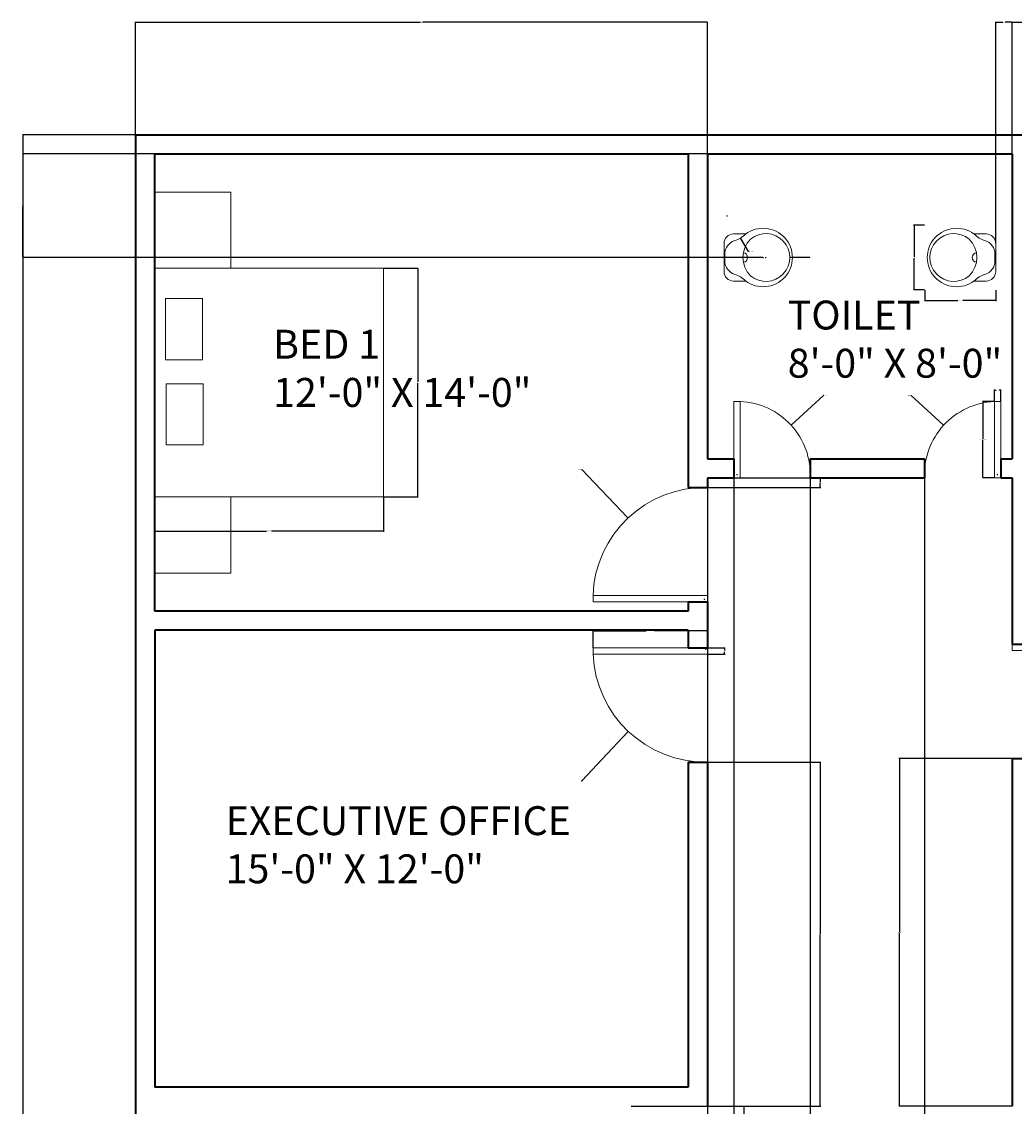
# Model space of a CAD drawing. Units: inches. Extents: x 4468 to 4972, y 2758 to 3538.
# Tile 3 of 4: x 4468 to 4781, y 3196 to 3538. Entities that reach past the tile are written whole.
import ezdxf

# ---------------------------------------------------------------- set-up
doc = ezdxf.new("R2010")
doc.units = ezdxf.units.IN
for name, color, linetype, lineweight in [('A-ANNO-DIMS', 2, 'Continuous', 18), ('A-AREA-IDEN', 7, 'Continuous', 18), ('A-DOOR', 4, 'Continuous', 18), ('A-FLOR-FIXT', 9, 'Continuous', 18), ('A-FURN', 8, 'Continuous', 15), ('A-WALL', 7, 'Continuous', 35)]:
    doc.layers.add(name, color=color, linetype=linetype, lineweight=lineweight)
doc.styles.get("Standard").update_dxf_attribs({"font": 'arial.ttf'})
doc.dimstyles.get("Standard").update_dxf_attribs({"dimtxt": 0.18, "dimasz": 0.18, "dimexe": 0.18, "dimexo": 0.0625, "dimgap": 0.09, "dimtad": 0, "dimtih": 1, "dimtoh": 1, "dimdec": 4, "dimzin": 0, "dimdsep": 46, "dimtxsty": 'Standard', "dimcen": 0.09, "dimadec": 0, "dimazin": 0, "dimtfac": 1, "dimtdec": 4, "dimtofl": 0, "dimtmove": 0, "dimatfit": 3, "dimfxl": 1, "dimtolj": 1, "dimtzin": 0, "dimarcsym": 0})

# ---------------------------------------------------------------- blocks, each defined once
blk = doc.blocks.new('A$C6EF51710')
at = {"linetype": 'ByBlock'}
for p, q in [((0.0508, 0.2843), (0.1169, 0.2843)), ((0, 0.0811), (0, 0.2335)), ((0.0041, 0.1392), (0.0041, 0.1755)), ((0.1169, 0.0303), (0.0508, 0.0303))]:
    blk.add_line(p, q, dxfattribs=at)
for centre, radius, start, end in [((0.2107, 0.1573), 0.1576, 232.89836, 127.10164), ((0.0508, 0.2335), 0.0508, 90, 180), ((0.0803, 0.1755), 0.0762, 107.10464, 180), ((0.0168, 0.3818), 0.1397, 287.10464, 315), ((0.2413, 0.1573), 0.1397, 135, 225), ((0.2254, 0.1573), 0.1289, 230.00836, 129.99164), ((0.1016, 0.1573), 0.0254, 275.21591, 84.78409), ((0.0803, 0.1392), 0.0762, 180, 252.89536), ((0.0508, 0.0811), 0.0508, 180, 270), ((0.0168, -0.0672), 0.1397, 45, 72.89536)]:
    blk.add_arc(centre, radius, start, end, dxfattribs=at)
blk = doc.blocks.new('DOOR-LEAF-36IN')
for p, q in [((0, 0), (0, 36)), ((0, 36), (2, 36)), ((2, 36), (2, 0)), ((2, 0), (0, 0))]:
    blk.add_line(p, q)
blk = doc.blocks.new('DOOR-LEAF-24IN')
for p, q in [((2, 24), (0, 24)), ((0, 24), (0, 0)), ((2, 0), (2, 24)), ((0, 0), (2, 0))]:
    blk.add_line(p, q)
blk = doc.blocks.new('BED-FRAME-72X72')
for p, q in [((0, 72), (0, 0)), ((0, 72), (72, 72)), ((0, 0), (72, 0))]:
    blk.add_line(p, q)
blk = doc.blocks.new('BED-PILLOW-PAIR')
for points in [[(0, 46.15), (11.65, 46.15), (11.65, 26.85), (0, 26.85)], [(0.18, 19.3), (11.83, 19.3), (11.83, 0), (0.18, 0)]]:
    blk.add_lwpolyline(points, close=True)
blk = doc.blocks.new('NIGHTSTAND-24X24')
blk.add_lwpolyline([(24, 24), (24, 0), (0, 0), (0, 24)], close=True)
blk = doc.blocks.new('*D17')
at = {"layer": 'A-ANNO-DIMS', "color": 0, "lineweight": -2, "transparency": 16777216}
for p, q in [((4648.18, 3340.62), (4648.18, 3346.13)), ((4648.36, 3345.95), (4664.89, 3345.95)), ((4684, 3345.95), (4667.46, 3345.95)), ((4684.18, 3340.62), (4684.18, 3346.13))]:
    blk.add_line(p, q, dxfattribs=at)
at = {"layer": 'A-ANNO-DIMS', "color": 0, "transparency": 16777216}
for points in [[(4648.36, 3345.98), (4648.36, 3345.92), (4648.18, 3345.95)], [(4684, 3345.98), (4684, 3345.92), (4684.18, 3345.95)]]:
    blk.add_solid(points, dxfattribs=at)
at = {"layer": 'Defpoints', "color": 0, "transparency": 16777216}
for p in [(4684.18, 3345.95), (4648.18, 3340.55), (4684.18, 3340.55)]:
    blk.add_point(p, dxfattribs=at)
at = {"layer": 'A-ANNO-DIMS', "color": 0, "transparency": 16777216, "insert": (4666.18, 3345.95), "char_height": 0.18, "attachment_point": 5}
blk.add_mtext('\\A1;DOOR LEAF 36 TYP.', dxfattribs=at)
blk = doc.blocks.new('*D18')
at = {"layer": 'A-ANNO-DIMS', "color": 0, "lineweight": -2, "transparency": 16777216}
for p, q in [((4684.24, 3340.55), (4689.76, 3340.55)), ((4684.24, 3338.55), (4689.76, 3338.55)), ((4689.58, 3340.37), (4689.58, 3339.73)), ((4689.58, 3338.73), (4689.58, 3339.37))]:
    blk.add_line(p, q, dxfattribs=at)
at = {"layer": 'A-ANNO-DIMS', "color": 0, "transparency": 16777216}
for points in [[(4689.55, 3340.37), (4689.61, 3340.37), (4689.58, 3340.55)], [(4689.55, 3338.73), (4689.61, 3338.73), (4689.58, 3338.55)]]:
    blk.add_solid(points, dxfattribs=at)
at = {"layer": 'Defpoints', "color": 0, "transparency": 16777216}
for p in [(4684.18, 3340.55), (4684.18, 3338.55), (4689.58, 3338.55)]:
    blk.add_point(p, dxfattribs=at)
at = {"layer": 'A-ANNO-DIMS', "color": 0, "transparency": 16777216, "insert": (4689.58, 3339.55), "char_height": 0.18, "attachment_point": 5}
blk.add_mtext('\\A1;2 TYP.', dxfattribs=at)
blk = doc.blocks.new('*D25')
at = {"layer": 'A-ANNO-DIMS', "color": 0, "lineweight": -2, "transparency": 16777216}
for p, q in [((4752.63, 3453.27), (4752.63, 3449.8)), ((4774.97, 3453.27), (4774.97, 3449.8)), ((4752.81, 3449.98), (4763.03, 3449.98)), ((4774.79, 3449.98), (4764.58, 3449.98))]:
    blk.add_line(p, q, dxfattribs=at)
at = {"layer": 'A-ANNO-DIMS', "color": 0, "transparency": 16777216}
for points in [[(4752.81, 3450.01), (4752.81, 3449.95), (4752.63, 3449.98)], [(4774.79, 3450.01), (4774.79, 3449.95), (4774.97, 3449.98)]]:
    blk.add_solid(points, dxfattribs=at)
at = {"layer": 'Defpoints', "color": 0, "transparency": 16777216}
for p in [(4752.63, 3453.33), (4774.97, 3453.33), (4752.63, 3449.98)]:
    blk.add_point(p, dxfattribs=at)
at = {"layer": 'A-ANNO-DIMS', "color": 0, "transparency": 16777216, "insert": (4763.8, 3449.98), "char_height": 0.18, "attachment_point": 5}
blk.add_mtext('\\A1;WC 22 TYP.', dxfattribs=at)
blk = doc.blocks.new('*D26')
at = {"layer": 'A-ANNO-DIMS', "color": 0, "lineweight": -2, "transparency": 16777216}
for p, q in [((4752.57, 3473.78), (4749.1, 3473.78)), ((4749.28, 3473.6), (4749.28, 3463.74)), ((4749.28, 3453.51), (4749.28, 3463.37)), ((4752.57, 3453.33), (4749.1, 3453.33))]:
    blk.add_line(p, q, dxfattribs=at)
at = {"layer": 'A-ANNO-DIMS', "color": 0, "transparency": 16777216}
for points in [[(4749.25, 3473.6), (4749.31, 3473.6), (4749.28, 3473.78)], [(4749.25, 3453.51), (4749.31, 3453.51), (4749.28, 3453.33)]]:
    blk.add_solid(points, dxfattribs=at)
at = {"layer": 'Defpoints', "color": 0, "transparency": 16777216}
for p in [(4749.28, 3473.78), (4752.63, 3473.78), (4752.63, 3453.33)]:
    blk.add_point(p, dxfattribs=at)
at = {"layer": 'A-ANNO-DIMS', "color": 0, "transparency": 16777216, "insert": (4749.28, 3463.55), "char_height": 0.18, "attachment_point": 5}
blk.add_mtext('\\A1;20 TYP.', dxfattribs=at)
blk = doc.blocks.new('*D29')
at = {"layer": 'A-ANNO-DIMS', "color": 0, "lineweight": -2, "transparency": 16777216}
for p, q in [((4774.49, 3418.16), (4770.77, 3418.16)), ((4770.95, 3417.98), (4770.95, 3406.34)), ((4770.95, 3394.34), (4770.95, 3405.98)), ((4774.49, 3394.16), (4770.77, 3394.16))]:
    blk.add_line(p, q, dxfattribs=at)
at = {"layer": 'A-ANNO-DIMS', "color": 0, "transparency": 16777216}
for points in [[(4770.92, 3417.98), (4770.98, 3417.98), (4770.95, 3418.16)], [(4770.92, 3394.34), (4770.98, 3394.34), (4770.95, 3394.16)]]:
    blk.add_solid(points, dxfattribs=at)
at = {"layer": 'Defpoints', "color": 0, "transparency": 16777216}
for p in [(4770.95, 3418.16), (4774.55, 3418.16), (4774.55, 3394.16)]:
    blk.add_point(p, dxfattribs=at)
at = {"layer": 'A-ANNO-DIMS', "color": 0, "transparency": 16777216, "insert": (4770.95, 3406.16), "char_height": 0.18, "attachment_point": 5}
blk.add_mtext('\\A1;DOOR LEAF 24 TYP.', dxfattribs=at)
blk = doc.blocks.new('*D30')
at = {"layer": 'A-ANNO-DIMS', "color": 0, "lineweight": -2, "transparency": 16777216}
for p, q in [((4774.55, 3418.22), (4774.55, 3421.94)), ((4774.73, 3421.76), (4775.09, 3421.76)), ((4776.37, 3421.76), (4776.01, 3421.76)), ((4776.55, 3418.22), (4776.55, 3421.94))]:
    blk.add_line(p, q, dxfattribs=at)
at = {"layer": 'A-ANNO-DIMS', "color": 0, "transparency": 16777216}
for points in [[(4774.73, 3421.79), (4774.73, 3421.73), (4774.55, 3421.76)], [(4776.37, 3421.79), (4776.37, 3421.73), (4776.55, 3421.76)]]:
    blk.add_solid(points, dxfattribs=at)
at = {"layer": 'Defpoints', "color": 0, "transparency": 16777216}
for p in [(4776.55, 3421.76), (4774.55, 3418.16), (4776.55, 3418.16)]:
    blk.add_point(p, dxfattribs=at)
at = {"layer": 'A-ANNO-DIMS', "color": 0, "transparency": 16777216, "insert": (4775.55, 3421.76), "char_height": 0.18, "attachment_point": 5}
blk.add_mtext('\\A1;2 TYP.', dxfattribs=at)
blk = doc.blocks.new('*D31')
at = {"layer": 'A-ANNO-DIMS', "color": 0, "lineweight": -2, "transparency": 16777216}
for p, q in [((4510.18, 3388.1), (4510.18, 3377.18)), ((4582.18, 3388.1), (4582.18, 3377.18)), ((4510.36, 3377.36), (4545.36, 3377.36)), ((4582, 3377.36), (4546.99, 3377.36))]:
    blk.add_line(p, q, dxfattribs=at)
at = {"layer": 'A-ANNO-DIMS', "color": 0, "transparency": 16777216}
for points in [[(4510.36, 3377.39), (4510.36, 3377.33), (4510.18, 3377.36)], [(4582, 3377.39), (4582, 3377.33), (4582.18, 3377.36)]]:
    blk.add_solid(points, dxfattribs=at)
at = {"layer": 'Defpoints', "color": 0, "transparency": 16777216}
for p in [(4510.18, 3388.16), (4582.18, 3388.16), (4510.18, 3377.36)]:
    blk.add_point(p, dxfattribs=at)
at = {"layer": 'A-ANNO-DIMS', "color": 0, "transparency": 16777216, "insert": (4546.18, 3377.36), "char_height": 0.18, "attachment_point": 5}
blk.add_mtext('\\A1;BED 72 TYP.', dxfattribs=at)
blk = doc.blocks.new('*D32')
at = {"layer": 'A-ANNO-DIMS', "color": 0, "lineweight": -2, "transparency": 16777216}
for p, q in [((4582.24, 3460.16), (4593.16, 3460.16)), ((4592.98, 3459.98), (4592.98, 3424.34)), ((4592.98, 3388.34), (4592.98, 3423.98)), ((4582.24, 3388.16), (4593.16, 3388.16))]:
    blk.add_line(p, q, dxfattribs=at)
at = {"layer": 'A-ANNO-DIMS', "color": 0, "transparency": 16777216}
for points in [[(4592.95, 3459.98), (4593.01, 3459.98), (4592.98, 3460.16)], [(4592.95, 3388.34), (4593.01, 3388.34), (4592.98, 3388.16)]]:
    blk.add_solid(points, dxfattribs=at)
at = {"layer": 'Defpoints', "color": 0, "transparency": 16777216}
for p in [(4582.18, 3460.16), (4582.18, 3388.16), (4592.98, 3388.16)]:
    blk.add_point(p, dxfattribs=at)
at = {"layer": 'A-ANNO-DIMS', "color": 0, "transparency": 16777216, "insert": (4592.98, 3424.16), "char_height": 0.18, "attachment_point": 5}
blk.add_mtext('\\A1;72 TYP.', dxfattribs=at)
blk = doc.blocks.new('*D38')
at = {"layer": 'A-ANNO-DIMS', "color": 0, "lineweight": -2, "transparency": 16777216}
for p, q in [((4504.11, 3502.16), (4468.5, 3502.16)), ((4468.68, 3501.98), (4468.68, 3148.34)), ((4468.68, 2794.34), (4468.68, 3147.98)), ((4780.11, 2794.16), (4468.5, 2794.16))]:
    blk.add_line(p, q, dxfattribs=at)
at = {"layer": 'A-ANNO-DIMS', "color": 0, "transparency": 16777216}
for points in [[(4468.65, 3501.98), (4468.71, 3501.98), (4468.68, 3502.16)], [(4468.65, 2794.34), (4468.71, 2794.34), (4468.68, 2794.16)]]:
    blk.add_solid(points, dxfattribs=at)
at = {"layer": 'Defpoints', "color": 0, "transparency": 16777216}
for p in [(4468.68, 3502.16), (4504.18, 3502.16), (4780.18, 2794.16)]:
    blk.add_point(p, dxfattribs=at)
at = {"layer": 'A-ANNO-DIMS', "color": 0, "transparency": 16777216, "insert": (4468.68, 3148.16), "char_height": 0.18, "attachment_point": 5}
blk.add_mtext('\\A1;708', dxfattribs=at)
blk = doc.blocks.new('*D39')
at = {"layer": 'A-ANNO-DIMS', "color": 0, "lineweight": -2, "transparency": 16777216}
for p, q in [((4504.18, 3502.22), (4504.18, 3537.84)), ((4504.36, 3537.66), (4593.9, 3537.66)), ((4684, 3537.66), (4594.46, 3537.66)), ((4684.18, 3496.22), (4684.18, 3537.84))]:
    blk.add_line(p, q, dxfattribs=at)
at = {"layer": 'A-ANNO-DIMS', "color": 0, "transparency": 16777216}
for points in [[(4504.36, 3537.69), (4504.36, 3537.63), (4504.18, 3537.66)], [(4684, 3537.69), (4684, 3537.63), (4684.18, 3537.66)]]:
    blk.add_solid(points, dxfattribs=at)
at = {"layer": 'Defpoints', "color": 0, "transparency": 16777216}
for p in [(4684.18, 3537.66), (4504.18, 3502.16), (4684.18, 3496.16)]:
    blk.add_point(p, dxfattribs=at)
at = {"layer": 'A-ANNO-DIMS', "color": 0, "transparency": 16777216, "insert": (4594.18, 3537.66), "char_height": 0.18, "attachment_point": 5}
blk.add_mtext('\\A1;180', dxfattribs=at)
blk = doc.blocks.new('*D40')
at = {"layer": 'A-ANNO-DIMS', "color": 0, "lineweight": -2, "transparency": 16777216}
for p, q in [((4780.18, 3496.22), (4780.18, 3537.84)), ((4780.36, 3537.66), (4857.9, 3537.66)), ((4936, 3537.66), (4858.46, 3537.66)), ((4936.18, 3502.22), (4936.18, 3537.84))]:
    blk.add_line(p, q, dxfattribs=at)
at = {"layer": 'A-ANNO-DIMS', "color": 0, "transparency": 16777216}
for points in [[(4780.36, 3537.69), (4780.36, 3537.63), (4780.18, 3537.66)], [(4936, 3537.69), (4936, 3537.63), (4936.18, 3537.66)]]:
    blk.add_solid(points, dxfattribs=at)
at = {"layer": 'Defpoints', "color": 0, "transparency": 16777216}
for p in [(4936.18, 3537.66), (4936.18, 3502.16), (4780.18, 3496.16)]:
    blk.add_point(p, dxfattribs=at)
at = {"layer": 'A-ANNO-DIMS', "color": 0, "transparency": 16777216, "insert": (4858.18, 3537.66), "char_height": 0.18, "attachment_point": 5}
blk.add_mtext('\\A1;156', dxfattribs=at)
blk = doc.blocks.new('*D50')
at = {"layer": 'A-ANNO-DIMS', "color": 0, "lineweight": -2, "transparency": 16777216}
for p, q in [((4660.24, 3196.16), (4695.86, 3196.16)), ((4695.68, 3195.98), (4695.68, 3136.34)), ((4695.68, 3076.34), (4695.68, 3135.98)), ((4660.24, 3076.16), (4695.86, 3076.16))]:
    blk.add_line(p, q, dxfattribs=at)
at = {"layer": 'A-ANNO-DIMS', "color": 0, "transparency": 16777216}
for points in [[(4695.65, 3195.98), (4695.71, 3195.98), (4695.68, 3196.16)], [(4695.65, 3076.34), (4695.71, 3076.34), (4695.68, 3076.16)]]:
    blk.add_solid(points, dxfattribs=at)
at = {"layer": 'Defpoints', "color": 0, "transparency": 16777216}
for p in [(4660.18, 3196.16), (4660.18, 3076.16), (4695.68, 3076.16)]:
    blk.add_point(p, dxfattribs=at)
at = {"layer": 'A-ANNO-DIMS', "color": 0, "transparency": 16777216, "insert": (4695.68, 3136.16), "char_height": 0.18, "attachment_point": 5}
blk.add_mtext('\\A1;120', dxfattribs=at)
blk = doc.blocks.new('*D61')
at = {"layer": 'A-ANNO-DIMS', "color": 0, "lineweight": -2, "transparency": 16777216}
for p, q in [((4684.24, 3304.55), (4719.86, 3304.55)), ((4719.68, 3304.37), (4719.68, 3250.54)), ((4719.68, 3196.34), (4719.68, 3250.17)), ((4684.24, 3196.16), (4719.86, 3196.16))]:
    blk.add_line(p, q, dxfattribs=at)
at = {"layer": 'A-ANNO-DIMS', "color": 0, "transparency": 16777216}
for points in [[(4719.65, 3304.37), (4719.71, 3304.37), (4719.68, 3304.55)], [(4719.65, 3196.34), (4719.71, 3196.34), (4719.68, 3196.16)]]:
    blk.add_solid(points, dxfattribs=at)
at = {"layer": 'Defpoints', "color": 0, "transparency": 16777216}
for p in [(4684.18, 3304.55), (4684.18, 3196.16), (4719.68, 3196.16)]:
    blk.add_point(p, dxfattribs=at)
at = {"layer": 'A-ANNO-DIMS', "color": 0, "transparency": 16777216, "insert": (4719.68, 3250.36), "char_height": 0.18, "attachment_point": 5}
blk.add_mtext('\\A1;108.4', dxfattribs=at)
blk = doc.blocks.new('*D62')
at = {"layer": 'A-ANNO-DIMS', "color": 0, "lineweight": -2, "transparency": 16777216}
for p, q in [((4780.11, 3305.72), (4744.5, 3305.72)), ((4744.68, 3305.54), (4744.68, 3251.12)), ((4744.68, 3196.34), (4744.68, 3250.76)), ((4780.11, 3196.16), (4744.5, 3196.16))]:
    blk.add_line(p, q, dxfattribs=at)
at = {"layer": 'A-ANNO-DIMS', "color": 0, "transparency": 16777216}
for points in [[(4744.65, 3305.54), (4744.71, 3305.54), (4744.68, 3305.72)], [(4744.65, 3196.34), (4744.71, 3196.34), (4744.68, 3196.16)]]:
    blk.add_solid(points, dxfattribs=at)
at = {"layer": 'Defpoints', "color": 0, "transparency": 16777216}
for p in [(4744.68, 3305.72), (4780.18, 3305.72), (4780.18, 3196.16)]:
    blk.add_point(p, dxfattribs=at)
at = {"layer": 'A-ANNO-DIMS', "color": 0, "transparency": 16777216, "insert": (4744.68, 3250.94), "char_height": 0.18, "attachment_point": 5}
blk.add_mtext('\\A1;109.56', dxfattribs=at)
blk = doc.blocks.new('*D63')
at = {"layer": 'A-ANNO-DIMS', "color": 0, "lineweight": -2, "transparency": 16777216}
for p, q in [((4684.24, 3394.16), (4719.86, 3394.16)), ((4719.68, 3393.98), (4719.68, 3392.79)), ((4684.24, 3391.05), (4719.86, 3391.05)), ((4719.68, 3391.23), (4719.68, 3392.42))]:
    blk.add_line(p, q, dxfattribs=at)
at = {"layer": 'A-ANNO-DIMS', "color": 0, "transparency": 16777216}
for points in [[(4719.65, 3393.98), (4719.71, 3393.98), (4719.68, 3394.16)], [(4719.65, 3391.23), (4719.71, 3391.23), (4719.68, 3391.05)]]:
    blk.add_solid(points, dxfattribs=at)
at = {"layer": 'Defpoints', "color": 0, "transparency": 16777216}
for p in [(4684.18, 3394.16), (4684.18, 3391.05), (4719.68, 3391.05)]:
    blk.add_point(p, dxfattribs=at)
at = {"layer": 'A-ANNO-DIMS', "color": 0, "transparency": 16777216, "insert": (4719.68, 3392.6), "char_height": 0.18, "attachment_point": 5}
blk.add_mtext('\\A1;3.108', dxfattribs=at)
blk = doc.blocks.new('*D66')
at = {"layer": 'A-ANNO-DIMS', "color": 0, "lineweight": -2, "transparency": 16777216}
for p, q in [((4684.18, 3394.1), (4684.18, 2758.48)), ((4692.55, 3394.1), (4692.55, 2758.48)), ((4684.36, 2758.66), (4687.97, 2758.66)), ((4692.37, 2758.66), (4688.76, 2758.66))]:
    blk.add_line(p, q, dxfattribs=at)
at = {"layer": 'A-ANNO-DIMS', "color": 0, "transparency": 16777216}
for points in [[(4684.36, 2758.69), (4684.36, 2758.63), (4684.18, 2758.66)], [(4692.37, 2758.69), (4692.37, 2758.63), (4692.55, 2758.66)]]:
    blk.add_solid(points, dxfattribs=at)
at = {"layer": 'Defpoints', "color": 0, "transparency": 16777216}
for p in [(4684.18, 3394.16), (4692.55, 3394.16), (4692.55, 2758.66)]:
    blk.add_point(p, dxfattribs=at)
at = {"layer": 'A-ANNO-DIMS', "color": 0, "transparency": 16777216, "insert": (4688.36, 2758.66), "char_height": 0.18, "attachment_point": 5}
blk.add_mtext('\\A1;8.375', dxfattribs=at)
blk = doc.blocks.new('*D67')
at = {"layer": 'A-ANNO-DIMS', "color": 0, "lineweight": -2, "transparency": 16777216}
for p, q in [((4716.55, 3394.1), (4716.55, 2758.48)), ((4752.55, 3394.1), (4752.55, 2758.48)), ((4716.73, 2758.66), (4734.33, 2758.66)), ((4752.37, 2758.66), (4734.77, 2758.66))]:
    blk.add_line(p, q, dxfattribs=at)
at = {"layer": 'A-ANNO-DIMS', "color": 0, "transparency": 16777216}
for points in [[(4716.73, 2758.69), (4716.73, 2758.63), (4716.55, 2758.66)], [(4752.37, 2758.69), (4752.37, 2758.63), (4752.55, 2758.66)]]:
    blk.add_solid(points, dxfattribs=at)
at = {"layer": 'Defpoints', "color": 0, "transparency": 16777216}
for p in [(4716.55, 3394.16), (4752.55, 3394.16), (4752.55, 2758.66)]:
    blk.add_point(p, dxfattribs=at)
at = {"layer": 'A-ANNO-DIMS', "color": 0, "transparency": 16777216, "insert": (4734.55, 2758.66), "char_height": 0.18, "attachment_point": 5}
blk.add_mtext('\\A1;36', dxfattribs=at)
blk = doc.blocks.new('*D68')
at = {"layer": 'A-ANNO-DIMS', "color": 0, "lineweight": -2, "transparency": 16777216}
for p, q in [((4774.97, 3468.07), (4774.97, 3537.84)), ((4775.15, 3537.66), (4777.18, 3537.66)), ((4780, 3537.66), (4777.97, 3537.66)), ((4780.18, 3496.22), (4780.18, 3537.84))]:
    blk.add_line(p, q, dxfattribs=at)
at = {"layer": 'A-ANNO-DIMS', "color": 0, "transparency": 16777216}
for points in [[(4775.15, 3537.69), (4775.15, 3537.63), (4774.97, 3537.66)], [(4780, 3537.69), (4780, 3537.63), (4780.18, 3537.66)]]:
    blk.add_solid(points, dxfattribs=at)
at = {"layer": 'Defpoints', "color": 0, "transparency": 16777216}
for p in [(4780.18, 3537.66), (4780.18, 3496.16), (4774.97, 3468.01)]:
    blk.add_point(p, dxfattribs=at)
at = {"layer": 'A-ANNO-DIMS', "color": 0, "transparency": 16777216, "insert": (4777.57, 3537.66), "char_height": 0.18, "attachment_point": 5}
blk.add_mtext('\\A1;5.207', dxfattribs=at)
blk = doc.blocks.new('*D69')
at = {"layer": 'A-ANNO-DIMS', "color": 0, "lineweight": -2, "transparency": 16777216}
for p, q in [((4684.11, 3496.16), (4468.5, 3496.16)), ((4468.68, 3495.98), (4468.68, 3480.04)), ((4468.68, 3463.73), (4468.68, 3479.67)), ((4701.68, 3463.55), (4468.5, 3463.55))]:
    blk.add_line(p, q, dxfattribs=at)
at = {"layer": 'A-ANNO-DIMS', "color": 0, "transparency": 16777216}
for points in [[(4468.65, 3495.98), (4468.71, 3495.98), (4468.68, 3496.16)], [(4468.65, 3463.73), (4468.71, 3463.73), (4468.68, 3463.55)]]:
    blk.add_solid(points, dxfattribs=at)
at = {"layer": 'Defpoints', "color": 0, "transparency": 16777216}
for p in [(4468.68, 3496.16), (4684.18, 3496.16), (4701.75, 3463.55)]:
    blk.add_point(p, dxfattribs=at)
at = {"layer": 'A-ANNO-DIMS', "color": 0, "transparency": 16777216, "insert": (4468.68, 3479.86), "char_height": 0.18, "attachment_point": 5}
blk.add_mtext('\\A1;32.604', dxfattribs=at)
blk = doc.blocks.new('*D75')
at = {"layer": 'A-ANNO-DIMS', "color": 0, "lineweight": -2, "transparency": 16777216}
for p, q in [((4683.65, 3340.15), (4683.83, 3340.15)), ((4683.74, 3340.06), (4683.74, 3340.24)), ((4644.63, 3298.74), (4659.17, 3314.14)), ((4644.45, 3298.74), (4644.63, 3298.74))]:
    blk.add_line(p, q, dxfattribs=at)
at = {"layer": 'A-ANNO-DIMS', "color": 0, "transparency": 16777216}
blk.add_solid([(4659.15, 3314.16), (4659.19, 3314.12), (4659.29, 3314.27)], dxfattribs=at)
at = {"layer": 'Defpoints', "color": 0, "transparency": 16777216}
for p in [(4683.74, 3340.15), (4659.29, 3314.27)]:
    blk.add_point(p, dxfattribs=at)
at = {"layer": 'A-ANNO-DIMS', "color": 0, "transparency": 16777216, "insert": (4644.04, 3298.74), "char_height": 0.18, "attachment_point": 5}
blk.add_mtext('\\A1;R35.6', dxfattribs=at)
blk = doc.blocks.new('*D77')
at = {"layer": 'A-ANNO-DIMS', "color": 0, "lineweight": -2, "transparency": 16777216}
for p, q in [((4644.51, 3396.8), (4644.69, 3396.8)), ((4644.69, 3396.8), (4659.04, 3381.6)), ((4683.2, 3355.93), (4683.38, 3355.93)), ((4683.29, 3355.84), (4683.29, 3356.02))]:
    blk.add_line(p, q, dxfattribs=at)
at = {"layer": 'A-ANNO-DIMS', "color": 0, "transparency": 16777216}
blk.add_solid([(4659.07, 3381.62), (4659.02, 3381.58), (4659.17, 3381.47)], dxfattribs=at)
at = {"layer": 'Defpoints', "color": 0, "transparency": 16777216}
for p in [(4659.17, 3381.47), (4683.29, 3355.93)]:
    blk.add_point(p, dxfattribs=at)
at = {"layer": 'A-ANNO-DIMS', "color": 0, "transparency": 16777216, "insert": (4643.96, 3396.8), "char_height": 0.18, "attachment_point": 5}
blk.add_mtext('\\A1;R35.134', dxfattribs=at)
blk = doc.blocks.new('*D81')
at = {"layer": 'A-ANNO-DIMS', "color": 0, "lineweight": -2, "transparency": 16777216}
for p, q in [((4748.22, 3420.05), (4748.4, 3420.05)), ((4748.4, 3420.05), (4758.44, 3410.84)), ((4775.45, 3395.17), (4775.63, 3395.17)), ((4775.54, 3395.08), (4775.54, 3395.26))]:
    blk.add_line(p, q, dxfattribs=at)
at = {"layer": 'A-ANNO-DIMS', "color": 0, "transparency": 16777216}
blk.add_solid([(4758.46, 3410.86), (4758.42, 3410.82), (4758.58, 3410.72)], dxfattribs=at)
at = {"layer": 'Defpoints', "color": 0, "transparency": 16777216}
for p in [(4758.58, 3410.72), (4775.54, 3395.17)]:
    blk.add_point(p, dxfattribs=at)
at = {"layer": 'A-ANNO-DIMS', "color": 0, "transparency": 16777216, "insert": (4747.76, 3420.05), "char_height": 0.18, "attachment_point": 5}
blk.add_mtext('\\A1;R23.01', dxfattribs=at)
blk = doc.blocks.new('*D82')
at = {"layer": 'A-ANNO-DIMS', "color": 0, "lineweight": -2, "transparency": 16777216}
for p, q in [((4720.7, 3420.04), (4710.67, 3410.85)), ((4720.88, 3420.04), (4720.7, 3420.04)), ((4693.51, 3395.2), (4693.69, 3395.2)), ((4693.6, 3395.11), (4693.6, 3395.29))]:
    blk.add_line(p, q, dxfattribs=at)
at = {"layer": 'A-ANNO-DIMS', "color": 0, "transparency": 16777216}
blk.add_solid([(4710.65, 3410.87), (4710.69, 3410.83), (4710.54, 3410.73)], dxfattribs=at)
at = {"layer": 'Defpoints', "color": 0, "transparency": 16777216}
for p in [(4710.54, 3410.73), (4693.6, 3395.2)]:
    blk.add_point(p, dxfattribs=at)
at = {"layer": 'A-ANNO-DIMS', "color": 0, "transparency": 16777216, "insert": (4721.43, 3420.04), "char_height": 0.18, "attachment_point": 5}
blk.add_mtext('\\A1;R22.974', dxfattribs=at)
blk = doc.blocks.new('*D83')
at = {"layer": 'A-ANNO-DIMS', "color": 0, "lineweight": -2, "transparency": 16777216}
for p, q in [((4701.66, 3463.55), (4701.84, 3463.55)), ((4701.75, 3463.46), (4701.75, 3463.64)), ((4716.49, 3463.55), (4711.14, 3463.55))]:
    blk.add_line(p, q, dxfattribs=at)
at = {"layer": 'A-ANNO-DIMS', "color": 0, "transparency": 16777216}
blk.add_solid([(4711.14, 3463.58), (4711.14, 3463.52), (4710.96, 3463.55)], dxfattribs=at)
at = {"layer": 'Defpoints', "color": 0, "transparency": 16777216}
for p in [(4701.75, 3463.55), (4710.96, 3463.55)]:
    blk.add_point(p, dxfattribs=at)
at = {"layer": 'A-ANNO-DIMS', "color": 0, "transparency": 16777216, "insert": (4716.97, 3463.55), "char_height": 0.18, "attachment_point": 5}
blk.add_mtext('\\A1;R9.216', dxfattribs=at)
blk = doc.blocks.new('*D84')
at = {"layer": 'A-ANNO-DIMS', "color": 0, "lineweight": -2, "transparency": 16777216}
for p, q in [((4690.32, 3476.68), (4690.5, 3476.68)), ((4690.41, 3476.59), (4690.41, 3476.77)), ((4697.15, 3465.48), (4694.72, 3469.53)), ((4697.33, 3465.48), (4697.15, 3465.48))]:
    blk.add_line(p, q, dxfattribs=at)
at = {"layer": 'A-ANNO-DIMS', "color": 0, "transparency": 16777216}
blk.add_solid([(4694.74, 3469.54), (4694.69, 3469.51), (4694.63, 3469.68)], dxfattribs=at)
at = {"layer": 'Defpoints', "color": 0, "transparency": 16777216}
for p in [(4690.41, 3476.68), (4694.63, 3469.68)]:
    blk.add_point(p, dxfattribs=at)
at = {"layer": 'A-ANNO-DIMS', "color": 0, "transparency": 16777216, "insert": (4698.01, 3465.48), "char_height": 0.18, "attachment_point": 5}
blk.add_mtext('\\A1;3X R8.167', dxfattribs=at)
blk = doc.blocks.new('*D85')
at = {"layer": 'A-ANNO-DIMS', "color": 0, "lineweight": -2, "transparency": 16777216}
for p, q in [((4702.52, 3463.55), (4702.7, 3463.55)), ((4702.61, 3463.46), (4702.61, 3463.64)), ((4714.67, 3463.55), (4710.33, 3463.55))]:
    blk.add_line(p, q, dxfattribs=at)
at = {"layer": 'A-ANNO-DIMS', "color": 0, "transparency": 16777216}
blk.add_solid([(4710.33, 3463.58), (4710.33, 3463.52), (4710.15, 3463.55)], dxfattribs=at)
at = {"layer": 'Defpoints', "color": 0, "transparency": 16777216}
for p in [(4702.61, 3463.55), (4710.15, 3463.55)]:
    blk.add_point(p, dxfattribs=at)
at = {"layer": 'A-ANNO-DIMS', "color": 0, "transparency": 16777216, "insert": (4715.15, 3463.55), "char_height": 0.18, "attachment_point": 5}
blk.add_mtext('\\A1;R7.538', dxfattribs=at)

msp = doc.modelspace()

# ---------------------------------------------------------------- linework, layer by layer
at = {"layer": 'A-DOOR'}
for centre, radius, start, end in [((4693.5998, 3395.2035), 22.9744, 357.392222, 87.628672), ((4775.5392, 3395.1685), 23.011, 92.462906, 182.5162), ((4683.2915, 3355.9273), 35.1341, 88.558455, 178.168391), ((4683.7366, 3340.1471), 35.597, 182.567009, 270.706145), ((4781.5553, 3340.3178), 34.6252, 267.715973, 359.010873)]:
    msp.add_arc(centre, radius, start, end, dxfattribs=at)
at = {"layer": 'A-WALL'}
for p, q in [((4504.1753, 3502.1582), (4936.1753, 3502.1582)), ((4504.1753, 3502.1582), (4504.1753, 2896.1582)), ((4510.1753, 3496.1582), (4678.1753, 3496.1582)), ((4510.1753, 3352.1582), (4510.1753, 3496.1582)), ((4678.1753, 3496.1582), (4678.1753, 3391.0502)), ((4684.1753, 3496.1582), (4684.1753, 3400.1582)), ((4684.1753, 3496.1582), (4780.1753, 3496.1582)), ((4780.1753, 3496.1582), (4780.1753, 3400.1582)), ((4684.1753, 3400.1582), (4692.5504, 3400.1582)), ((4692.5504, 3400.1582), (4692.5504, 3394.1582)), ((4716.5504, 3400.1582), (4716.5504, 3394.1582)), ((4716.5504, 3400.1582), (4752.5504, 3400.1582)), ((4752.5504, 3400.1582), (4752.5504, 3394.1582)), ((4776.5504, 3400.1582), (4776.5504, 3394.1582)), ((4776.5504, 3400.1582), (4780.1753, 3400.1582)), ((4684.1753, 3394.1582), (4692.5504, 3394.1582)), ((4684.1753, 3394.1582), (4684.1753, 3391.0502)), ((4716.5504, 3394.1582), (4752.5504, 3394.1582)), ((4776.5504, 3394.1582), (4780.1753, 3394.1582)), ((4780.1753, 3394.1582), (4780.1753, 3341.7201)), ((4678.1753, 3391.0502), (4684.1753, 3391.0502)), ((4678.1753, 3352.1582), (4510.1753, 3352.1582)), ((4678.1753, 3355.0502), (4684.1753, 3355.0502)), ((4678.1753, 3355.0502), (4678.1753, 3352.1582)), ((4684.1753, 3355.0502), (4684.1753, 3340.5528)), ((4678.1753, 3346.1582), (4510.1753, 3346.1582)), ((4510.1753, 3346.1582), (4510.1753, 3202.1582)), ((4678.1753, 3346.1582), (4678.1753, 3340.5528)), ((4780.1753, 3341.7201), (4786.1753, 3341.7201)), ((4678.1753, 3340.5528), (4684.1753, 3340.5528)), ((4678.1753, 3304.5528), (4684.1753, 3304.5528)), ((4678.1753, 3304.5528), (4678.1753, 3202.1582)), ((4684.1753, 3304.5528), (4684.1753, 3196.1582)), ((4780.1753, 3305.7201), (4786.1753, 3305.7201)), ((4780.1753, 3305.7201), (4780.1753, 3196.1582)), ((4678.1753, 3202.1582), (4510.1753, 3202.1582))]:
    msp.add_line(p, q, dxfattribs=at)

# ---------------------------------------------------------------- block references
at = {"layer": 'A-DOOR'}
for name, p, rotation in [('DOOR-LEAF-24IN', (4694.5504, 3418.1582), 180), ('DOOR-LEAF-36IN', (4684.1753, 3355.0502), 90.00000000000146), ('DOOR-LEAF-36IN', (4780.1753, 3341.7201), 270), ('DOOR-LEAF-36IN', (4648.1753, 3340.5528), 270)]:
    msp.add_blockref(name, p, dxfattribs=dict(at, rotation=rotation))
msp.add_blockref('DOOR-LEAF-24IN', (4774.5504, 3394.1582), dxfattribs=at)
at = {"layer": 'A-FLOR-FIXT', "yscale": 58.46424994274177, "zscale": 58.46424994274177}
for p, xscale in [((4689.4301, 3454.3562), 58.46424994274177), ((4774.9686, 3454.3562), -58.46424994274177)]:
    msp.add_blockref('A$C6EF51710', p, dxfattribs=dict(at, xscale=xscale))
at = {"layer": 'A-FURN'}
for name, p in [('NIGHTSTAND-24X24', (4510.1753, 3460.1582)), ('BED-PILLOW-PAIR', (4513.6225, 3404.4965)), ('NIGHTSTAND-24X24', (4510.1753, 3364.1582))]:
    msp.add_blockref(name, p, dxfattribs=at)
at = {"layer": 'A-FURN', "rotation": 180}
msp.add_blockref('BED-FRAME-72X72', (4582.1753, 3460.1582), dxfattribs=at)

# ---------------------------------------------------------------- texts
at = {"layer": 'A-AREA-IDEN', "char_height": 9.103585, "attachment_point": 1}
for s, insert in [('TOILET\\P8\'-0" X 8\'-0"', (4709.4759, 3449.9735)), ('BED 1\\P12\'-0" X 14\'-0"', (4547.4483, 3440.78)), ('EXECUTIVE OFFICE\\P15\'-0" X 12\'-0"', (4532.4973, 3290.6973))]:
    msp.add_mtext_dynamic_manual_height_columns(s, width=327.642018, gutter_width=45.5179, heights=[0], dxfattribs=dict(at, insert=insert))

# ---------------------------------------------------------------- dimensions: what is measured, and where the dimension line sits
at = {"layer": 'A-ANNO-DIMS'}
for base, p1, p2, override, picture, middle in [((4684.1753, 3537.6582), (4504.1753, 3502.1582), (4684.1753, 3496.1582), {"dimdec": 0, "dimlfac": 1, "dimrnd": 0, "dimzin": 0, "dimdsep": 46, "dimlunit": 2}, '*D39', (4594.1753, 3537.6582)), ((4780.1753, 3537.6582), (4774.9686, 3468.0092), (4780.1753, 3496.1582), {"dimdec": 3, "dimlfac": 1, "dimrnd": 0, "dimzin": 0, "dimdsep": 46, "dimlunit": 2}, '*D68', (4777.572, 3537.6582)), ((4936.1753, 3537.6582), (4780.1753, 3496.1582), (4936.1753, 3502.1582), {"dimdec": 0, "dimlfac": 1, "dimrnd": 0, "dimzin": 0, "dimdsep": 46, "dimlunit": 2}, '*D40', (4858.1753, 3537.6582)), ((4692.5504, 2758.6582), (4684.1753, 3394.1582), (4692.5504, 3394.1582), {"dimdec": 3, "dimlfac": 1, "dimrnd": 0, "dimzin": 0, "dimdsep": 46, "dimlunit": 2}, '*D66', (4688.3629, 2758.6582)), ((4752.5504, 2758.6582), (4716.5504, 3394.1582), (4752.5504, 3394.1582), {"dimdec": 0, "dimlfac": 1, "dimrnd": 0, "dimzin": 0, "dimdsep": 46, "dimlunit": 2}, '*D67', (4734.5504, 2758.6582))]:
    dim = msp.add_linear_dim(base=base, p1=p1, p2=p2, dimstyle='Standard', override=override, dxfattribs=at)
    dim.commit()
    dim.dimension.update_dxf_attribs({"geometry": picture, "text_midpoint": middle})
for base, p1, p2, angle, override, picture, middle in [((4468.6753, 3502.1582), (4780.1753, 2794.1582), (4504.1753, 3502.1582), 90, {"dimdec": 0, "dimlfac": 1, "dimrnd": 0, "dimzin": 0, "dimdsep": 46, "dimlunit": 2}, '*D38', (4468.6753, 3148.1582)), ((4468.6753, 3496.1582), (4701.7466, 3463.5543), (4684.1753, 3496.1582), 90, {"dimdec": 3, "dimlfac": 1, "dimrnd": 0, "dimzin": 0, "dimdsep": 46, "dimlunit": 2}, '*D69', (4468.6753, 3479.8562)), ((4719.6753, 3391.0502), (4684.1753, 3394.1582), (4684.1753, 3391.0502), 270, {"dimdec": 3, "dimlfac": 1, "dimrnd": 0, "dimzin": 0, "dimdsep": 46, "dimlunit": 2}, '*D63', (4719.6753, 3392.6042)), ((4719.6753, 3196.1582), (4684.1753, 3304.5528), (4684.1753, 3196.1582), 270, {"dimdec": 1, "dimlfac": 1, "dimrnd": 0, "dimzin": 0, "dimdsep": 46, "dimlunit": 2}, '*D61', (4719.6753, 3250.3555)), ((4744.6753, 3305.7201), (4780.1753, 3196.1582), (4780.1753, 3305.7201), 90, {"dimdec": 2, "dimlfac": 1, "dimrnd": 0, "dimzin": 0, "dimdsep": 46, "dimlunit": 2}, '*D62', (4744.6753, 3250.9391)), ((4695.6753, 3076.1582), (4660.1753, 3196.1582), (4660.1753, 3076.1582), 270, {"dimdec": 0, "dimlfac": 1, "dimrnd": 0, "dimzin": 0, "dimdsep": 46, "dimlunit": 2}, '*D50', (4695.6753, 3136.1582))]:
    dim = msp.add_linear_dim(base=base, p1=p1, p2=p2, angle=angle, dimstyle='Standard', override=override, dxfattribs=at)
    dim.commit()
    dim.dimension.update_dxf_attribs({"geometry": picture, "text_midpoint": middle})
dim = msp.add_radius_dim(center=(4690.412, 3476.6799), mpoint=(4694.625, 3469.6829), text='3X <>', dimstyle='Standard', override={"dimdec": 3, "dimlfac": 1, "dimrnd": 0, "dimzin": 0, "dimdsep": 46, "dimlunit": 2}, dxfattribs=at)
dim.commit()
dim.dimension.update_dxf_attribs({"geometry": '*D84', "text_midpoint": (4698.0061, 3465.4848), "dimtype": 164})
for base, p1, p2, angle, text, picture, middle in [((4749.2838, 3473.7773), (4752.634, 3453.3313), (4752.634, 3473.7773), 90, '<> TYP.', '*D26', (4749.2838, 3463.5543)), ((4592.9753, 3388.1582), (4582.1753, 3460.1582), (4582.1753, 3388.1582), 270, '<> TYP.', '*D32', (4592.9753, 3424.1582)), ((4752.634, 3449.9811), (4774.9686, 3453.3313), (4752.634, 3453.3313), 180, 'WC <> TYP.', '*D25', (4763.8013, 3449.9811)), ((4770.9504, 3418.1582), (4774.5504, 3394.1582), (4774.5504, 3418.1582), 90, 'DOOR LEAF <> TYP.', '*D29', (4770.9504, 3406.1582)), ((4510.1753, 3377.3582), (4582.1753, 3388.1582), (4510.1753, 3388.1582), 180, 'BED <> TYP.', '*D31', (4546.1753, 3377.3582)), ((4689.5753, 3338.5528), (4684.1753, 3340.5528), (4684.1753, 3338.5528), 270, '<> TYP.', '*D18', (4689.5753, 3339.5528))]:
    dim = msp.add_linear_dim(base=base, p1=p1, p2=p2, angle=angle, text=text, dimstyle='Standard', override={"dimdec": 0, "dimlfac": 1, "dimrnd": 0, "dimzin": 0, "dimdsep": 46, "dimlunit": 2}, dxfattribs=at)
    dim.commit()
    dim.dimension.update_dxf_attribs({"geometry": picture, "text_midpoint": middle})
for center, mpoint, override, picture, middle in [((4701.7466, 3463.5543), (4710.9625, 3463.554), {"dimdec": 3, "dimlfac": 1, "dimrnd": 0, "dimzin": 0, "dimdsep": 46, "dimlunit": 2}, '*D83', (4716.4921, 3463.5538)), ((4702.6069, 3463.5543), (4710.145, 3463.554), {"dimdec": 3, "dimlfac": 1, "dimrnd": 0, "dimzin": 0, "dimdsep": 46, "dimlunit": 2}, '*D85', (4714.6679, 3463.5538)), ((4693.5998, 3395.2035), (4710.5352, 3410.7282), {"dimdec": 3, "dimlfac": 1, "dimrnd": 0, "dimzin": 0, "dimdsep": 46, "dimlunit": 2}, '*D82', (4721.4258, 3420.043)), ((4775.5392, 3395.1685), (4758.577, 3410.718), {"dimdec": 2, "dimlfac": 1, "dimrnd": 0, "dimzin": 0, "dimdsep": 46, "dimlunit": 2}, '*D81', (4747.7571, 3420.0478)), ((4683.2915, 3355.9273), (4659.1677, 3381.4703), {"dimdec": 3, "dimlfac": 1, "dimrnd": 0, "dimzin": 0, "dimdsep": 46, "dimlunit": 2}, '*D77', (4643.9641, 3396.7962)), ((4683.7366, 3340.1471), (4659.2948, 3314.2677), {"dimdec": 1, "dimlfac": 1, "dimrnd": 0, "dimzin": 0, "dimdsep": 46, "dimlunit": 2}, '*D75', (4644.0398, 3298.7401))]:
    dim = msp.add_radius_dim(center=center, mpoint=mpoint, dimstyle='Standard', override=override, dxfattribs=at)
    dim.commit()
    dim.dimension.update_dxf_attribs({"geometry": picture, "text_midpoint": middle, "dimtype": 164})
for base, p1, p2, text, picture, middle in [((4776.5504, 3421.7582), (4774.5504, 3418.1582), (4776.5504, 3418.1582), '<> TYP.', '*D30', (4775.5504, 3421.7582)), ((4684.1753, 3345.9528), (4648.1753, 3340.5528), (4684.1753, 3340.5528), 'DOOR LEAF <> TYP.', '*D17', (4666.1753, 3345.9528))]:
    dim = msp.add_linear_dim(base=base, p1=p1, p2=p2, text=text, dimstyle='Standard', override={"dimdec": 0, "dimlfac": 1, "dimrnd": 0, "dimzin": 0, "dimdsep": 46, "dimlunit": 2}, dxfattribs=at)
    dim.commit()
    dim.dimension.update_dxf_attribs({"geometry": picture, "text_midpoint": middle})

doc.saveas('drawing.dxf')
